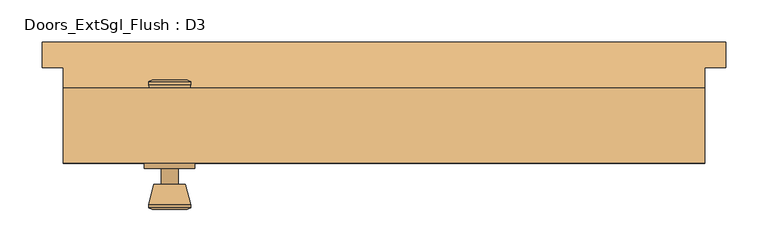
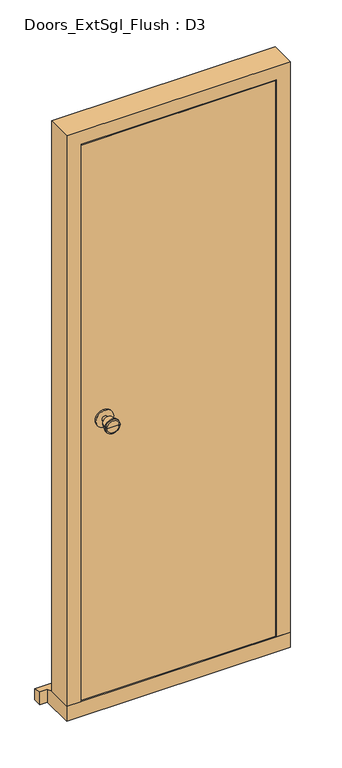
"""IFC4 building model written with IfcOpenShell, lengths in millimetres: door geometry, Doors_ExtSgl_Flush : D3."""

from ifc_helpers import new_model, si_unit, point, frame, frame_2d, origin, place, context, project, spatial, polyline, circle_curve, trimmed, segment, composite_curve, outline, extrude, faceted_brep, source, transform, mapped, element, save
from ifc_brep_helpers import plane_surface, cylinder_surface, revolved_surface, advanced_brep


def doors_extsgl_flush_d3_b5fe9048(model_context):
    return source(origin(), model_context, "Body", "SolidModel", [
        advanced_brep(
        [(-254.5, -95.3112, 1050.0), (-244.5, -95.3112, 1050.0), (-264.5, -95.3112, 1050.0), (-234.0241324, -144.3112, 1050.0), (-254.5, -144.3112, 1050.0), (-274.9758676, -144.3112, 1050.0), (-229.5, -142.4833319, 1050.0), (-279.5, -142.4833319, 1050.0), (-229.5, -139.0196537, 1050.0), (-279.5, -139.0196537, 1050.0), (-235.863764, -114.3112, 1050.0), (-273.136236, -114.3112, 1050.0), (-244.5, -114.3112, 1050.0), (-264.5, -114.3112, 1050.0)],
        [
            (0, 1),
            (1, 2, circle_curve(frame((-254.5, -95.3112, 1050.0), z_axis=(0.0, 1.0, 0.0), x_axis=(-1.0, 0.0, 0.0)), 10.0)),
            (2, 0),
            (2, 1, circle_curve(frame((-254.5, -95.3112, 1050.0), z_axis=(0.0, 1.0, 0.0), x_axis=(-1.0, 0.0, 0.0)), 10.0)),
            (3, 4),
            (4, 5),
            (5, 3, circle_curve(frame((-254.5, -144.3112, 1050.0), z_axis=(0.0, -1.0, 0.0), x_axis=(-1.0, 0.0, 0.0)), 20.4758676)),
            (3, 5, circle_curve(frame((-254.5, -144.3112, 1050.0), z_axis=(0.0, -1.0, 0.0), x_axis=(-1.0, 0.0, 0.0)), 20.4758676)),
            (6, 3),
            (5, 7),
            (7, 6, circle_curve(frame((-254.5, -142.4833319, 1050.0), z_axis=(0.0, -1.0, 0.0), x_axis=(-1.0, 0.0, 0.0)), 25.0)),
            (6, 7, circle_curve(frame((-254.5, -142.4833319, 1050.0), z_axis=(0.0, -1.0, 0.0), x_axis=(-1.0, 0.0, 0.0)), 25.0)),
            (8, 6),
            (7, 9),
            (9, 8, circle_curve(frame((-254.5, -139.0196537, 1050.0), z_axis=(0.0, -1.0, 0.0), x_axis=(-1.0, 0.0, 0.0)), 25.0)),
            (8, 9, circle_curve(frame((-254.5, -139.0196537, 1050.0), z_axis=(0.0, -1.0, 0.0), x_axis=(-1.0, 0.0, 0.0)), 25.0)),
            (10, 8),
            (9, 11),
            (11, 10, circle_curve(frame((-254.5, -114.3112, 1050.0), z_axis=(0.0, -1.0, 0.0), x_axis=(-1.0, 0.0, 0.0)), 18.636236)),
            (10, 11, circle_curve(frame((-254.5, -114.3112, 1050.0), z_axis=(0.0, -1.0, 0.0), x_axis=(-1.0, 0.0, 0.0)), 18.636236)),
            (12, 10),
            (11, 13),
            (13, 12, circle_curve(frame((-254.5, -114.3112, 1050.0), z_axis=(0.0, -1.0, 0.0), x_axis=(-1.0, 0.0, 0.0)), 10.0)),
            (12, 13, circle_curve(frame((-254.5, -114.3112, 1050.0), z_axis=(0.0, -1.0, 0.0), x_axis=(-1.0, 0.0, 0.0)), 10.0)),
            (1, 12),
            (13, 2),
        ],
        [
            plane_surface(frame((-254.5, -95.3112, 1050.0), z_axis=(0.0, 1.0, 0.0), x_axis=(-1.0, 0.0, 0.0))),
            plane_surface(frame((-254.5, -144.3112, 1050.0), z_axis=(0.0, -1.0, 0.0), x_axis=(-1.0, 0.0, 0.0))),
            revolved_surface(polyline([(-274.9758676, -144.3112, 1050.0), (-279.5, -142.4833319, 1050.0)]), (-254.5, -95.3112, 1050.0), (0.0, 1.0, 0.0)),
            cylinder_surface(frame((-254.5, -95.3112, 1050.0), z_axis=(0.0, 1.0, 0.0), x_axis=(-1.0, 0.0, 0.0)), 25.0),
            revolved_surface(polyline([(-279.5, -139.0196537, 1050.0), (-273.136236, -114.3112, 1050.0)]), (-254.5, -95.3112, 1050.0), (0.0, 1.0, 0.0)),
            plane_surface(frame((-254.5, -114.3112, 1050.0), z_axis=(0.0, 1.0, 0.0), x_axis=(-1.0, 0.0, 0.0))),
            cylinder_surface(frame((-254.5, -95.3112, 1050.0), z_axis=(0.0, 1.0, 0.0), x_axis=(-1.0, 0.0, 0.0)), 10.0),
        ],
        [
            (0, [[1, 2, 3]]),
            (0, [[-3, 4, -1]]),
            (1, [[5, 6, 7]]),
            (1, [[-6, -5, 8]]),
            (2, [[9, -7, 10, 11]]),
            (2, [[-10, -8, -9, 12]]),
            (3, [[13, -11, 14, 15]]),
            (3, [[-14, -12, -13, 16]]),
            (4, [[17, -15, 18, 19]]),
            (4, [[-18, -16, -17, 20]]),
            (5, [[21, -19, 22, 23]]),
            (5, [[-22, -20, -21, 24]]),
            (6, [[25, -23, 26, -2]]),
            (6, [[-26, -24, -25, -4]]),
        ],
    ),
        extrude(outline(composite_curve([segment(trimmed(circle_curve(frame_2d((1050.0, -254.5)), 30.0), [point((1050.0, -284.5))], [point((1050.0, -224.5))], False, "CARTESIAN"), True, "CONTINUOUS"), segment(trimmed(circle_curve(frame_2d((1050.0, -254.5)), 30.0), [point((1050.0, -224.5))], [point((1050.0, -284.5))], False, "CARTESIAN"), True, "CONTINUOUS")], self_intersect=False)), frame((0.0, -95.3112, 0.0), z_axis=(0.0, 1.0, 0.0), x_axis=(0.0, 0.0, 1.0)), (0.0, 0.0, 1.0), 6.0),
        advanced_brep(
        [(-254.5, -39.3112, 1050.0), (-264.5, -39.3112, 1050.0), (-244.5, -39.3112, 1050.0), (-234.0241324, 9.6888, 1050.0), (-274.9758676, 9.6888, 1050.0), (-254.5, 9.6888, 1050.0), (-229.5, 7.8609319, 1050.0), (-279.5, 7.8609319, 1050.0), (-229.5, 4.3972537, 1050.0), (-279.5, 4.3972537, 1050.0), (-235.863764, -20.3112, 1050.0), (-273.136236, -20.3112, 1050.0), (-244.5, -20.3112, 1050.0), (-264.5, -20.3112, 1050.0)],
        [
            (0, 1),
            (1, 2, circle_curve(frame((-254.5, -39.3112, 1050.0), z_axis=(0.0, -1.0, 0.0), x_axis=(-1.0, 0.0, 0.0)), 10.0)),
            (2, 0),
            (2, 1, circle_curve(frame((-254.5, -39.3112, 1050.0), z_axis=(0.0, -1.0, 0.0), x_axis=(-1.0, 0.0, 0.0)), 10.0)),
            (3, 4, circle_curve(frame((-254.5, 9.6888, 1050.0), z_axis=(0.0, 1.0, 0.0), x_axis=(-1.0, 0.0, 0.0)), 20.4758676)),
            (4, 5),
            (5, 3),
            (4, 3, circle_curve(frame((-254.5, 9.6888, 1050.0), z_axis=(0.0, 1.0, 0.0), x_axis=(-1.0, 0.0, 0.0)), 20.4758676)),
            (6, 7, circle_curve(frame((-254.5, 7.8609319, 1050.0), z_axis=(0.0, 1.0, 0.0), x_axis=(-1.0, 0.0, 0.0)), 25.0)),
            (7, 4),
            (3, 6),
            (7, 6, circle_curve(frame((-254.5, 7.8609319, 1050.0), z_axis=(0.0, 1.0, 0.0), x_axis=(-1.0, 0.0, 0.0)), 25.0)),
            (8, 9, circle_curve(frame((-254.5, 4.3972537, 1050.0), z_axis=(0.0, 1.0, 0.0), x_axis=(-1.0, 0.0, 0.0)), 25.0)),
            (9, 7),
            (6, 8),
            (9, 8, circle_curve(frame((-254.5, 4.3972537, 1050.0), z_axis=(0.0, 1.0, 0.0), x_axis=(-1.0, 0.0, 0.0)), 25.0)),
            (10, 11, circle_curve(frame((-254.5, -20.3112, 1050.0), z_axis=(0.0, 1.0, 0.0), x_axis=(-1.0, 0.0, 0.0)), 18.636236)),
            (11, 9),
            (8, 10),
            (11, 10, circle_curve(frame((-254.5, -20.3112, 1050.0), z_axis=(0.0, 1.0, 0.0), x_axis=(-1.0, 0.0, 0.0)), 18.636236)),
            (12, 13, circle_curve(frame((-254.5, -20.3112, 1050.0), z_axis=(0.0, 1.0, 0.0), x_axis=(-1.0, 0.0, 0.0)), 10.0)),
            (13, 11),
            (10, 12),
            (13, 12, circle_curve(frame((-254.5, -20.3112, 1050.0), z_axis=(0.0, 1.0, 0.0), x_axis=(-1.0, 0.0, 0.0)), 10.0)),
            (1, 13),
            (12, 2),
        ],
        [
            plane_surface(frame((-254.5, -39.3112, 1050.0), z_axis=(0.0, -1.0, 0.0), x_axis=(-1.0, 0.0, 0.0))),
            plane_surface(frame((-254.5, 9.6888, 1050.0), z_axis=(0.0, 1.0, 0.0), x_axis=(-1.0, 0.0, 0.0))),
            revolved_surface(polyline([(-274.9758676, 9.6888, 1050.0), (-279.5, 7.8609319, 1050.0)]), (-254.5, -39.3112, 1050.0), (0.0, -1.0, 0.0)),
            cylinder_surface(frame((-254.5, -39.3112, 1050.0), z_axis=(0.0, -1.0, 0.0), x_axis=(-1.0, 0.0, 0.0)), 25.0),
            revolved_surface(polyline([(-279.5, 4.3972537, 1050.0), (-273.136236, -20.3112, 1050.0)]), (-254.5, -39.3112, 1050.0), (0.0, -1.0, 0.0)),
            plane_surface(frame((-254.5, -20.3112, 1050.0), z_axis=(0.0, -1.0, 0.0), x_axis=(-1.0, 0.0, 0.0))),
            cylinder_surface(frame((-254.5, -39.3112, 1050.0), z_axis=(0.0, -1.0, 0.0), x_axis=(-1.0, 0.0, 0.0)), 10.0),
        ],
        [
            (0, [[1, 2, 3]]),
            (0, [[-3, 4, -1]]),
            (1, [[5, 6, 7]]),
            (1, [[8, -7, -6]]),
            (2, [[9, 10, -5, 11]]),
            (2, [[12, -11, -8, -10]]),
            (3, [[13, 14, -9, 15]]),
            (3, [[16, -15, -12, -14]]),
            (4, [[17, 18, -13, 19]]),
            (4, [[20, -19, -16, -18]]),
            (5, [[21, 22, -17, 23]]),
            (5, [[24, -23, -20, -22]]),
            (6, [[-2, 25, -21, 26]]),
            (6, [[-4, -26, -24, -25]]),
        ],
    ),
        extrude(outline(composite_curve([segment(trimmed(circle_curve(frame_2d((1050.0, -254.5)), 30.0), [point((1050.0, -284.5))], [point((1050.0, -224.5))], False, "CARTESIAN"), True, "CONTINUOUS"), segment(trimmed(circle_curve(frame_2d((1050.0, -254.5)), 30.0), [point((1050.0, -224.5))], [point((1050.0, -284.5))], False, "CARTESIAN"), True, "CONTINUOUS")], self_intersect=False)), frame((0.0, -45.3112, 0.0), z_axis=(0.0, 1.0, 0.0), x_axis=(0.0, 0.0, 1.0)), (0.0, 0.0, 1.0), 6.0),
        faceted_brep([(310.5, -0.3112, 54.5), (381.0, -0.3112, 54.5), (381.0, -89.3112, 54.5), (332.5, -89.3112, 54.5), (332.5, -42.3112, 54.5), (310.5, -42.3112, 54.5), (310.5, -0.3112, 2039.5), (-310.5, -0.3112, 2039.5), (-310.5, -0.3112, 54.5), (-381.0, -0.3112, 54.5), (-381.0, -0.3112, 2110.0), (381.0, -0.3112, 2110.0), (381.0, -89.3112, 2110.0), (-381.0, -89.3112, 2110.0), (-381.0, -89.3112, 54.5), (-332.5, -89.3112, 54.5), (-332.5, -89.3112, 2061.5), (332.5, -89.3112, 2061.5), (332.5, -42.3112, 2061.5), (-332.5, -42.3112, 2061.5), (-332.5, -42.3112, 54.5), (-310.5, -42.3112, 54.5), (-310.5, -42.3112, 2039.5), (310.5, -42.3112, 2039.5)], [[[0, 1, 2, 3, 4, 5]], [[1, 0, 6, 7, 8, 9, 10, 11]], [[2, 1, 11, 12]], [[3, 2, 12, 13, 14, 15, 16, 17]], [[4, 3, 17, 18]], [[5, 4, 18, 19, 20, 21, 22, 23]], [[0, 5, 23, 6]], [[7, 22, 21, 8]], [[8, 21, 20, 15, 14, 9]], [[13, 10, 9, 14]], [[19, 16, 15, 20]], [[12, 11, 10, 13]], [[18, 17, 16, 19]], [[6, 23, 22, 7]]]),
        extrude(outline(polyline([(329.5, -89.3112), (-330.4250294, -89.3112), (-330.4250294, -45.3112), (329.5, -45.3112), (329.5, -89.3112)])), frame((0.0, 0.0, 58.5), z_axis=(0.0, 0.0, 1.0), x_axis=(1.0, 0.0, 0.0)), (0.0, 0.0, 1.0), 2000.0),
        faceted_brep([(406.0, 54.6888, 0.0), (406.0, 54.6888, 38.5947221), (406.0, 24.6888, 47.2703282), (406.0, 24.6888, 0.0), (-406.0, 54.6888, 38.5947221), (-406.0, 54.6888, 0.0), (-406.0, 24.6888, 0.0), (-406.0, 24.6888, 47.2703282), (381.0, 24.6888, 0.0), (381.0, -89.3112, 0.0), (-381.0, -89.3112, 0.0), (-381.0, 24.6888, 0.0), (-381.0, 24.6888, 47.2703282), (-381.0, -0.3112, 54.5), (381.0, -0.3112, 54.5), (381.0, 24.6888, 47.2703282), (-381.0, -89.3112, 54.5), (381.0, -89.3112, 54.5)], [[[0, 1, 2, 3]], [[4, 5, 6, 7]], [[5, 0, 3, 8, 9, 10, 11, 6]], [[1, 0, 5, 4]], [[1, 4, 7, 12, 13, 14, 15, 2]], [[13, 16, 17, 14]], [[16, 10, 9, 17]], [[12, 11, 10, 16, 13]], [[11, 12, 7, 6]], [[8, 15, 14, 17, 9]], [[15, 8, 3, 2]]]),
    ])


if __name__ == "__main__":
    model = new_model("IFC4")
    model_context = context("Model", 3, world=origin())
    ifc_project = project(units=[si_unit("LENGTHUNIT", "METRE", prefix="MILLI")], contexts=[model_context])
    site = spatial("IfcSite", under=ifc_project)
    building = spatial("IfcBuilding", under=site)
    placement = place(None, origin())
    doors_extsgl_flush_d3_shape = doors_extsgl_flush_d3_b5fe9048(model_context)
    element("IfcDoor", 1, ObjectType="Doors_ExtSgl_Flush : D3", at=placement, inside=building, context=model_context, shape_type="MappedRepresentation", body=[
        mapped(doors_extsgl_flush_d3_shape, transform((0.0, 0.0, 0.0), x_axis=(1.0, 0.0, 0.0), y_axis=(0.0, 1.0, 0.0), z_axis=(0.0, 0.0, 1.0))),
    ])
    save(model, "model.ifc")

# Revit data of these elements
# Type "Doors_ExtSgl_Flush : D3"
#   Type Mark = "51"
#   Type Comments = "External Single"
#   Operation = "SingleSwingRight"
#   Construction Type Id = "MDOOR"
#   Keynote = "L20"
#   Analytic Construction = "Metal"
#   Wrap Layers (Int) from Ext = 177.5 mm
#   Wrap Layers (Ext) from Ext = 102.5 mm
#   Thickness = 44 mm
#   Rough Width = 762 mm
#   Rough Height = 2110 mm
#   O/A Frame Width = 64 mm
#   Heat Transfer Coefficient (U) = 3.7021 W/(m²·K)
#   Handle Z Distance = 1050 mm
#   FrameWidth = 42 mm
#   FrameOffset - External = 25 mm
#   FrameDepth = 89 mm
#   Door Panel Width = 659 mm
#   Door Panel Thickness = 44 mm
#   Door Panel Height = 2000 mm
#   Cill Thickness = 54.5 mm
#   Cill Projection = 30 mm
#   Handle X Distance = 75 mm
#   Height = 2110 mm
#   Structural Tolerance = 6.5 mm
#   Tolerance = 3 mm
#   Undercut = 4 mm
#   Width = 762 mm
#   Cill Extension = 25 mm
#   Cavity Closer Width = 50 mm
#   Cavity Closer Offset from Ext = 102.5 mm
#   Cavity Closer Depth = 85 mm
#   Vis - Ironmongery = yes
#   Vis - Cavity Closers = yes
#   Define Thermal Properties by = 1
#   Function = 1
#   Material Door = Door - Panel
#   Material Frame = Door - Frame/Mullion
#   Material Ironmongery = Door - Handle
#   Visual Light Transmittance = 0
#   Solar Heat Gain Coefficient = 0
#   Wall Closure = (empty or 0)
# Element 1 (IfcDoor, "Doors_ExtSgl_Flush : D3")
#   Materials on its faces: "Door - Handle", "Door - Frame/Mullion", "Door - Panel"
# Materials
#   "Door - Panel": class "Wood", colour RGB 210 159 95, transparency 0, Keynote = "L20", Cost = 0
#   "Door - Frame/Mullion": class "Wood", colour RGB 212 179 113, transparency 0, Keynote = "L20", Cost = 0
#   "Door - Handle": colour RGB 0 0 0, transparency 0, Keynote = "P21", Cost = 0
